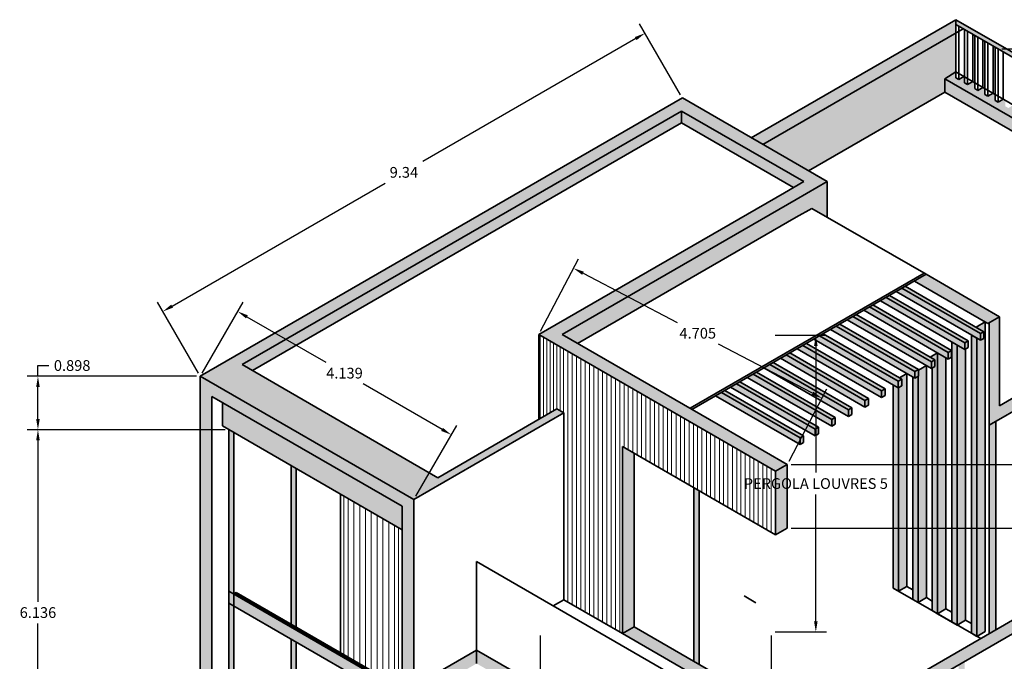
# Model space of a CAD drawing. Units: metres. Extents: x 26125 to 52281, y 14233 to 28508.
# Tile 3 of 4: x 26125.05 to 26141.57, y 14248.53 to 14259.3. Entities that reach past the tile are written whole.
import ezdxf

# ---------------------------------------------------------------- set-up
doc = ezdxf.new("R2010")
doc.units = ezdxf.units.M
for name, color, linetype, lineweight in [('A-ANNO-DIMS', 2, 'Continuous', 18), ('A-ELEV-CLAD', 30, 'Continuous', 13), ('A-ELEV-PATT', 32, 'Continuous', 13), ('A-WALL', 7, 'Continuous', 35), ('A-WALL-PATT', 9, 'Continuous', 13)]:
    doc.layers.add(name, color=color, linetype=linetype, lineweight=lineweight)
doc.styles.get("Standard").update_dxf_attribs({"font": 'arial.ttf'})
doc.dimstyles.get("Standard").update_dxf_attribs({"dimtxt": 0.18, "dimasz": 0.18, "dimexe": 0.18, "dimexo": 0.0625, "dimgap": 0.09, "dimtad": 0, "dimtih": 1, "dimtoh": 1, "dimdec": 4, "dimzin": 0, "dimdsep": 46, "dimtxsty": 'Standard', "dimcen": 0.09, "dimadec": 0, "dimazin": 0, "dimtfac": 1, "dimtdec": 4, "dimtofl": 0, "dimtmove": 0, "dimatfit": 3, "dimfxl": 1, "dimtolj": 1, "dimtzin": 0, "dimarcsym": 0})

# ---------------------------------------------------------------- blocks, each defined once
blk = doc.blocks.new('LINES')
for p, q in [((26133.777, 14254.006), (26133.777, 14252.604)), ((26133.833, 14253.974), (26133.833, 14252.637)), ((26133.889, 14253.942), (26133.889, 14252.669)), ((26133.945, 14253.91), (26133.945, 14252.701)), ((26134.001, 14253.877), (26134.001, 14252.733)), ((26134.057, 14253.845), (26134.057, 14252.766)), ((26134.112, 14253.813), (26134.112, 14252.738)), ((26134.168, 14253.781), (26134.168, 14252.706)), ((26134.241, 14253.739), (26134.241, 14249.53)), ((26134.314, 14253.697), (26134.314, 14249.488)), ((26134.386, 14253.655), (26134.386, 14249.446)), ((26134.459, 14253.613), (26134.459, 14249.404)), ((26134.532, 14253.571), (26134.532, 14249.362)), ((26134.604, 14253.529), (26134.604, 14249.32)), ((26134.677, 14253.487), (26134.677, 14249.278)), ((26134.75, 14253.445), (26134.75, 14249.236)), ((26134.822, 14253.403), (26134.822, 14249.194)), ((26134.895, 14253.361), (26134.895, 14249.152)), ((26134.968, 14253.319), (26134.968, 14249.111)), ((26135.04, 14253.277), (26135.04, 14249.069)), ((26135.113, 14253.235), (26135.113, 14249.027)), ((26135.186, 14253.193), (26135.186, 14252.124)), ((26135.258, 14253.151), (26135.258, 14252.082)), ((26135.331, 14253.109), (26135.331, 14252.04)), ((26135.404, 14253.067), (26135.404, 14251.998)), ((26135.477, 14253.025), (26135.477, 14251.956)), ((26135.549, 14252.983), (26135.549, 14251.914)), ((26135.622, 14252.941), (26135.622, 14251.872)), ((26135.695, 14252.899), (26135.695, 14251.83)), ((26135.767, 14252.857), (26135.767, 14251.788)), ((26135.84, 14252.815), (26135.84, 14251.746)), ((26135.913, 14252.774), (26135.913, 14251.704)), ((26135.985, 14252.732), (26135.985, 14251.662)), ((26136.058, 14252.69), (26136.058, 14251.62)), ((26136.131, 14252.648), (26136.131, 14251.578)), ((26136.203, 14252.606), (26136.203, 14251.536)), ((26136.276, 14252.564), (26136.276, 14251.494)), ((26136.349, 14252.522), (26136.349, 14251.452)), ((26136.421, 14252.48), (26136.421, 14251.41)), ((26136.494, 14252.438), (26136.494, 14251.368)), ((26136.567, 14252.396), (26136.567, 14251.326)), ((26136.639, 14252.354), (26136.639, 14251.284)), ((26136.712, 14252.312), (26136.712, 14251.242)), ((26136.785, 14252.27), (26136.785, 14251.2)), ((26136.857, 14252.228), (26136.857, 14251.158)), ((26136.93, 14252.186), (26136.93, 14251.116)), ((26137.003, 14252.144), (26137.003, 14251.074)), ((26137.076, 14252.102), (26137.076, 14251.033)), ((26137.148, 14252.06), (26137.148, 14250.991)), ((26137.221, 14252.018), (26137.221, 14250.949)), ((26137.294, 14251.976), (26137.294, 14250.907)), ((26137.366, 14251.934), (26137.366, 14250.865)), ((26137.439, 14251.892), (26137.439, 14250.823)), ((26137.512, 14251.85), (26137.512, 14250.781)), ((26137.584, 14251.808), (26137.584, 14250.739)), ((26137.657, 14251.766), (26137.657, 14250.697))]:
    blk.add_line(p, q)
blk = doc.blocks.new('*D8')
at = {"layer": 'A-ANNO-DIMS', "color": 0, "lineweight": -2, "transparency": 16777216}
for p, q in [((26137.719, 14254.006), (26138.584, 14254.006)), ((26138.404, 14253.826), (26138.404, 14251.7)), ((26138.404, 14249.207), (26138.404, 14251.333)), ((26137.719, 14249.027), (26138.584, 14249.027))]:
    blk.add_line(p, q, dxfattribs=at)
at = {"layer": 'A-ANNO-DIMS', "color": 0, "transparency": 16777216}
for points in [[(26138.374, 14253.826), (26138.434, 14253.826), (26138.404, 14254.006)], [(26138.374, 14249.207), (26138.434, 14249.207), (26138.404, 14249.027)]]:
    blk.add_solid(points, dxfattribs=at)
at = {"layer": 'Defpoints', "color": 0, "transparency": 16777216}
for p in [(26137.657, 14254.006), (26138.404, 14254.006), (26137.657, 14249.027)]:
    blk.add_point(p, dxfattribs=at)
at = {"layer": 'A-ANNO-DIMS', "color": 0, "transparency": 16777216, "insert": (26138.404, 14251.517), "char_height": 0.18, "attachment_point": 5}
blk.add_mtext('\\A1;PERGOLA LOUVRES 5', dxfattribs=at)
blk = doc.blocks.new('*D9')
at = {"layer": 'A-ANNO-DIMS', "color": 0, "lineweight": -2, "transparency": 16777216}
for p, q in [((26133.777, 14248.964), (26133.777, 14248.1)), ((26137.657, 14248.964), (26137.657, 14248.1)), ((26133.957, 14248.28), (26135.565, 14248.28)), ((26137.477, 14248.28), (26135.869, 14248.28))]:
    blk.add_line(p, q, dxfattribs=at)
at = {"layer": 'A-ANNO-DIMS', "color": 0, "transparency": 16777216}
for points in [[(26133.957, 14248.31), (26133.957, 14248.25), (26133.777, 14248.28)], [(26137.477, 14248.31), (26137.477, 14248.25), (26137.657, 14248.28)]]:
    blk.add_solid(points, dxfattribs=at)
at = {"layer": 'Defpoints', "color": 0, "transparency": 16777216}
for p in [(26133.777, 14249.027), (26137.657, 14249.027), (26137.657, 14248.28)]:
    blk.add_point(p, dxfattribs=at)
at = {"layer": 'A-ANNO-DIMS', "color": 0, "transparency": 16777216, "insert": (26135.717, 14248.28), "char_height": 0.18, "attachment_point": 5}
blk.add_mtext('\\A1;4', dxfattribs=at)
blk = doc.blocks.new('*D11')
at = {"layer": 'A-ANNO-DIMS', "color": 0, "lineweight": -2, "transparency": 16777216}
for p, q in [((26141.524, 14258.813), (26150.226, 14258.813)), ((26150.046, 14258.633), (26150.046, 14247.091)), ((26150.046, 14235.186), (26150.046, 14246.727)), ((26136.826, 14235.006), (26150.226, 14235.006))]:
    blk.add_line(p, q, dxfattribs=at)
at = {"layer": 'A-ANNO-DIMS', "color": 0, "transparency": 16777216}
for points in [[(26150.016, 14258.633), (26150.076, 14258.633), (26150.046, 14258.813)], [(26150.016, 14235.186), (26150.076, 14235.186), (26150.046, 14235.006)]]:
    blk.add_solid(points, dxfattribs=at)
at = {"layer": 'Defpoints', "color": 0, "transparency": 16777216}
for p in [(26141.462, 14258.813), (26150.046, 14258.813), (26136.763, 14235.006)]:
    blk.add_point(p, dxfattribs=at)
at = {"layer": 'A-ANNO-DIMS', "color": 0, "transparency": 16777216, "insert": (26150.046, 14246.909), "char_height": 0.18, "attachment_point": 5}
blk.add_mtext('\\A1;23.807', dxfattribs=at)
blk = doc.blocks.new('*D19')
at = {"layer": 'A-ANNO-DIMS', "color": 0, "lineweight": -2, "transparency": 16777216}
for p, q in [((26128.107, 14253.372), (26128.794, 14254.561)), ((26128.859, 14254.315), (26130.181, 14253.552)), ((26132.132, 14252.426), (26130.811, 14253.188)), ((26131.692, 14251.303), (26132.378, 14252.492))]:
    blk.add_line(p, q, dxfattribs=at)
at = {"layer": 'A-ANNO-DIMS', "color": 0, "transparency": 16777216}
for points in [[(26128.874, 14254.341), (26128.844, 14254.289), (26128.704, 14254.405)], [(26132.147, 14252.452), (26132.117, 14252.4), (26132.288, 14252.336)]]:
    blk.add_solid(points, dxfattribs=at)
at = {"layer": 'Defpoints', "color": 0, "transparency": 16777216}
for p in [(26128.076, 14253.318), (26132.288, 14252.336), (26131.66, 14251.249)]:
    blk.add_point(p, dxfattribs=at)
at = {"layer": 'A-ANNO-DIMS', "color": 0, "transparency": 16777216, "insert": (26130.496, 14253.37), "char_height": 0.18, "attachment_point": 5}
blk.add_mtext('\\A1;4.139', dxfattribs=at)
blk = doc.blocks.new('*D20')
at = {"layer": 'A-ANNO-DIMS', "color": 0, "lineweight": -2, "transparency": 16777216}
for p, q in [((26136.134, 14258.043), (26135.447, 14259.231)), ((26135.382, 14258.985), (26131.808, 14256.922)), ((26127.604, 14254.495), (26131.178, 14256.558)), ((26128.045, 14253.372), (26127.359, 14254.561))]:
    blk.add_line(p, q, dxfattribs=at)
at = {"layer": 'A-ANNO-DIMS', "color": 0, "transparency": 16777216}
for points in [[(26135.367, 14259.011), (26135.397, 14258.959), (26135.537, 14259.075)], [(26127.589, 14254.521), (26127.619, 14254.469), (26127.449, 14254.405)]]:
    blk.add_solid(points, dxfattribs=at)
at = {"layer": 'Defpoints', "color": 0, "transparency": 16777216}
for p in [(26135.537, 14259.075), (26136.165, 14257.988), (26128.076, 14253.318)]:
    blk.add_point(p, dxfattribs=at)
at = {"layer": 'A-ANNO-DIMS', "color": 0, "transparency": 16777216, "insert": (26131.493, 14256.74), "char_height": 0.18, "attachment_point": 5}
blk.add_mtext('\\A1;9.34', dxfattribs=at)
blk = doc.blocks.new('*D21')
at = {"layer": 'A-ANNO-DIMS', "color": 0, "lineweight": -2, "transparency": 16777216}
for p, q in [((26133.786, 14254.074), (26134.422, 14255.29)), ((26134.498, 14255.047), (26136.075, 14254.222)), ((26138.348, 14253.033), (26136.77, 14253.858)), ((26137.954, 14251.893), (26138.591, 14253.109))]:
    blk.add_line(p, q, dxfattribs=at)
at = {"layer": 'A-ANNO-DIMS', "color": 0, "transparency": 16777216}
for points in [[(26134.512, 14255.073), (26134.484, 14255.02), (26134.338, 14255.13)], [(26138.362, 14253.06), (26138.334, 14253.006), (26138.507, 14252.949)]]:
    blk.add_solid(points, dxfattribs=at)
at = {"layer": 'Defpoints', "color": 0, "transparency": 16777216}
for p in [(26133.757, 14254.018), (26138.507, 14252.949), (26137.925, 14251.837)]:
    blk.add_point(p, dxfattribs=at)
at = {"layer": 'A-ANNO-DIMS', "color": 0, "transparency": 16777216, "insert": (26136.423, 14254.04), "char_height": 0.18, "attachment_point": 5}
blk.add_mtext('\\A1;4.705', dxfattribs=at)
blk = doc.blocks.new('*D22')
at = {"layer": 'A-ANNO-DIMS', "color": 0, "lineweight": -2, "transparency": 16777216}
for p, q in [((26137.988, 14251.837), (26150.226, 14251.837)), ((26150.046, 14251.657), (26150.046, 14251.485)), ((26150.046, 14250.948), (26150.046, 14251.121)), ((26137.988, 14250.768), (26150.226, 14250.768))]:
    blk.add_line(p, q, dxfattribs=at)
at = {"layer": 'A-ANNO-DIMS', "color": 0, "transparency": 16777216}
for points in [[(26150.016, 14251.657), (26150.076, 14251.657), (26150.046, 14251.837)], [(26150.016, 14250.948), (26150.076, 14250.948), (26150.046, 14250.768)]]:
    blk.add_solid(points, dxfattribs=at)
at = {"layer": 'Defpoints', "color": 0, "transparency": 16777216}
for p in [(26137.925, 14251.837), (26137.925, 14250.768), (26150.046, 14250.768)]:
    blk.add_point(p, dxfattribs=at)
at = {"layer": 'A-ANNO-DIMS', "color": 0, "transparency": 16777216, "insert": (26150.046, 14251.303), "char_height": 0.18, "attachment_point": 5}
blk.add_mtext('\\A1;1.07', dxfattribs=at)
blk = doc.blocks.new('*D26')
at = {"layer": 'A-ANNO-DIMS', "color": 0, "lineweight": -2, "transparency": 16777216}
for p, q in [((26128.496, 14252.42), (26125.173, 14252.42)), ((26125.353, 14252.24), (26125.353, 14249.534)), ((26125.353, 14246.464), (26125.353, 14249.17)), ((26128.496, 14246.284), (26125.173, 14246.284))]:
    blk.add_line(p, q, dxfattribs=at)
at = {"layer": 'A-ANNO-DIMS', "color": 0, "transparency": 16777216}
for points in [[(26125.323, 14252.24), (26125.383, 14252.24), (26125.353, 14252.42)], [(26125.323, 14246.464), (26125.383, 14246.464), (26125.353, 14246.284)]]:
    blk.add_solid(points, dxfattribs=at)
at = {"layer": 'Defpoints', "color": 0, "transparency": 16777216}
for p in [(26125.353, 14252.42), (26128.558, 14252.42), (26128.558, 14246.284)]:
    blk.add_point(p, dxfattribs=at)
at = {"layer": 'A-ANNO-DIMS', "color": 0, "transparency": 16777216, "insert": (26125.353, 14249.352), "char_height": 0.18, "attachment_point": 5}
blk.add_mtext('\\A1;6.136', dxfattribs=at)
blk = doc.blocks.new('*D27')
at = {"layer": 'A-ANNO-DIMS', "color": 0, "lineweight": -2, "transparency": 16777216}
for p, q in [((26125.353, 14253.318), (26125.353, 14253.498)), ((26125.353, 14253.498), (26125.533, 14253.498)), ((26128.014, 14253.318), (26125.173, 14253.318)), ((26125.353, 14252.6), (26125.353, 14253.138)), ((26128.496, 14252.42), (26125.173, 14252.42))]:
    blk.add_line(p, q, dxfattribs=at)
at = {"layer": 'A-ANNO-DIMS', "color": 0, "transparency": 16777216}
for points in [[(26125.323, 14253.138), (26125.383, 14253.138), (26125.353, 14253.318)], [(26125.323, 14252.6), (26125.383, 14252.6), (26125.353, 14252.42)]]:
    blk.add_solid(points, dxfattribs=at)
at = {"layer": 'Defpoints', "color": 0, "transparency": 16777216}
for p in [(26125.353, 14253.318), (26128.076, 14253.318), (26128.558, 14252.42)]:
    blk.add_point(p, dxfattribs=at)
at = {"layer": 'A-ANNO-DIMS', "color": 0, "transparency": 16777216, "insert": (26125.927, 14253.498), "char_height": 0.18, "attachment_point": 5}
blk.add_mtext('\\A1;0.898', dxfattribs=at)

msp = doc.modelspace()

# ---------------------------------------------------------------- hatches: boundary and pattern name
at = {"layer": 'A-ELEV-PATT'}
h = msp.add_hatch(color=256, dxfattribs=at)
h.dxf.hatch_style = 1
h.paths.add_polyline_path([(26140.2525, 14255.0285), (26140.2206, 14255.0469), (26136.2935, 14252.7796), (26136.3254, 14252.7612)])
h = msp.add_hatch(color=256, dxfattribs=at)
h.dxf.hatch_style = 1
h.paths.add_polyline_path([(26137.9664, 14253.7086), (26137.9088, 14253.6753), (26139.2286, 14252.9133), (26139.2862, 14252.9466)])
h.paths.add_polyline_path([(26137.9088, 14253.6753), (26137.8118, 14253.6194), (26139.2286, 14252.8014), (26139.2286, 14252.9133)])
h.paths.add_polyline_path([(26139.2862, 14252.9466), (26139.2286, 14252.9133), (26139.2286, 14252.8014), (26139.2862, 14252.8347)])
h.paths.add_polyline_path([(26139.5077, 14253.0745), (26138.1879, 14253.8365), (26138.091, 14253.7805), (26139.5077, 14252.9626)])
h.paths.add_polyline_path([(26138.2456, 14253.8698), (26138.1879, 14253.8365), (26139.5077, 14253.0745), (26139.5654, 14253.1078)])
h.paths.add_polyline_path([(26139.5654, 14253.1078), (26139.5077, 14253.0745), (26139.5077, 14252.9626), (26139.5654, 14252.9959)])
h.paths.add_polyline_path([(26138.467, 14253.9977), (26138.3701, 14253.9417), (26139.7869, 14253.1237), (26139.7869, 14253.2357)])
h.paths.add_polyline_path([(26138.5247, 14254.0309), (26138.467, 14253.9977), (26139.7869, 14253.2357), (26139.8445, 14253.2689)])
h.paths.add_polyline_path([(26139.8445, 14253.2689), (26139.7869, 14253.2357), (26139.7869, 14253.1237), (26139.8445, 14253.157)])
h.paths.add_polyline_path([(26140.1237, 14253.4301), (26140.066, 14253.3968), (26140.066, 14253.2849), (26140.1237, 14253.3182)])
h.paths.add_polyline_path([(26138.8038, 14254.1921), (26138.7462, 14254.1588), (26140.066, 14253.3968), (26140.1237, 14253.4301)])
h.paths.add_polyline_path([(26138.7462, 14254.1588), (26138.6493, 14254.1029), (26140.066, 14253.2849), (26140.066, 14253.3968)])
h.paths.add_polyline_path([(26139.0253, 14254.32), (26138.9284, 14254.264), (26140.3451, 14253.4461), (26140.3451, 14253.558)])
h.paths.add_polyline_path([(26139.083, 14254.3533), (26139.0253, 14254.32), (26140.3451, 14253.558), (26140.4028, 14253.5913)])
h.paths.add_polyline_path([(26140.4028, 14253.5913), (26140.3451, 14253.558), (26140.3451, 14253.4461), (26140.4028, 14253.4793)])
h.paths.add_polyline_path([(26139.3045, 14254.4811), (26139.2075, 14254.4252), (26140.6243, 14253.6072), (26140.6243, 14253.7191)])
h.paths.add_polyline_path([(26139.3621, 14254.5144), (26139.3045, 14254.4811), (26140.6243, 14253.7191), (26140.6819, 14253.7524)])
h.paths.add_polyline_path([(26140.6819, 14253.7524), (26140.6243, 14253.7191), (26140.6243, 14253.6072), (26140.6819, 14253.6405)])
h.paths.add_polyline_path([(26139.5836, 14254.6423), (26139.4867, 14254.5863), (26140.9034, 14253.7684), (26140.9034, 14253.8803)])
h.paths.add_polyline_path([(26139.6412, 14254.6756), (26139.5836, 14254.6423), (26140.9034, 14253.8803), (26140.9611, 14253.9136)])
h.paths.add_polyline_path([(26140.9611, 14253.9136), (26140.9034, 14253.8803), (26140.9034, 14253.7684), (26140.9611, 14253.8017)])
h.paths.add_polyline_path([(26139.8476, 14254.7947), (26139.7506, 14254.7387), (26141.1674, 14253.9208), (26141.1674, 14254.0327)])
h.paths.add_polyline_path([(26139.9052, 14254.828), (26139.8476, 14254.7947), (26141.1674, 14254.0327), (26141.225, 14254.066)])
h.paths.add_polyline_path([(26141.225, 14254.066), (26141.1674, 14254.0327), (26141.1674, 14253.9208), (26141.225, 14253.9541)])
h = msp.add_hatch(color=256, dxfattribs=at)
h.dxf.hatch_style = 1
h.paths.add_polyline_path([(26141.2443, 14254.2299), (26141.0927, 14254.1424), (26141.225, 14254.066), (26141.225, 14253.9541), (26141.1674, 14253.9208), (26141.1045, 14253.9571), (26141.1045, 14249.1138), (26141.2443, 14249.0331)])
h.paths.add_polyline_path([(26141.2443, 14249.0331), (26141.1045, 14249.1138), (26141.1045, 14248.9523)])
h.paths.add_polyline_path([(26141.1045, 14253.9571), (26141.015, 14254.0088), (26141.015, 14249.004), (26141.1045, 14248.9523), (26141.1045, 14249.1138)])
h.paths.add_polyline_path([(26141.4248, 14252.5622), (26141.3093, 14252.4955), (26141.3093, 14248.9955), (26141.4248, 14249.0622)])
h.paths.add_polyline_path([(26140.9159, 14253.7756), (26140.9034, 14253.7684), (26140.7761, 14253.8419), (26140.7761, 14249.3033), (26140.9159, 14249.2226)])
h.paths.add_polyline_path([(26140.7761, 14253.8419), (26140.6854, 14253.8942), (26140.6854, 14249.1943), (26140.7761, 14249.1419)])
h.paths.add_polyline_path([(26140.9159, 14249.2226), (26140.7761, 14249.3033), (26140.7761, 14249.1419)])
h.paths.add_polyline_path([(26140.4478, 14249.4929), (26140.4478, 14249.3315), (26140.5876, 14249.4122)])
h.paths.add_polyline_path([(26140.5876, 14253.6284), (26140.4478, 14253.7091), (26140.4478, 14249.4929), (26140.5876, 14249.4122)])
h.paths.add_polyline_path([(26140.4478, 14253.7091), (26140.3232, 14253.6372), (26140.4028, 14253.5913), (26140.4028, 14253.4793), (26140.3571, 14253.4529), (26140.3571, 14249.3839), (26140.4478, 14249.3315), (26140.4478, 14249.4929)])
h.paths.add_polyline_path([(26140.2592, 14253.4957), (26140.1237, 14253.4174), (26140.1237, 14253.3182), (26140.1194, 14253.3157), (26140.1194, 14249.6825), (26140.2592, 14249.6018)])
h.paths.add_polyline_path([(26140.1194, 14253.3157), (26140.066, 14253.2849), (26140.0287, 14253.3064), (26140.0287, 14249.5735), (26140.1194, 14249.5211)])
h.paths.add_polyline_path([(26140.1194, 14249.6825), (26140.1194, 14249.5211), (26140.2592, 14249.6018)])
h = msp.add_hatch(color=256, dxfattribs=at)
h.dxf.hatch_style = 1
h.paths.add_polyline_path([(26136.8199, 14253.0467), (26136.723, 14252.9907), (26138.1397, 14252.1728), (26138.1397, 14252.2847)])
h.paths.add_polyline_path([(26136.8776, 14253.08), (26136.8199, 14253.0467), (26138.1397, 14252.2847), (26138.1974, 14252.318)])
h.paths.add_polyline_path([(26138.1974, 14252.318), (26138.1397, 14252.2847), (26138.1397, 14252.1728), (26138.1974, 14252.206)])
h.paths.add_polyline_path([(26137.0714, 14253.1918), (26136.9744, 14253.1359), (26138.3912, 14252.3179), (26138.3912, 14252.4298)])
h.paths.add_polyline_path([(26137.129, 14253.2251), (26137.0714, 14253.1918), (26138.3912, 14252.4298), (26138.4488, 14252.4631)])
h.paths.add_polyline_path([(26138.4488, 14252.4631), (26138.3912, 14252.4298), (26138.3912, 14252.3179), (26138.4488, 14252.3512)])
h.paths.add_polyline_path([(26137.3505, 14253.353), (26137.2536, 14253.2971), (26138.6703, 14252.4791), (26138.6703, 14252.591)])
h.paths.add_polyline_path([(26137.4081, 14253.3863), (26137.3505, 14253.353), (26138.6703, 14252.591), (26138.728, 14252.6243)])
h.paths.add_polyline_path([(26138.728, 14252.6243), (26138.6703, 14252.591), (26138.6703, 14252.4791), (26138.728, 14252.5124)])
h.paths.add_polyline_path([(26137.6296, 14253.5142), (26137.5327, 14253.4582), (26138.9495, 14252.6403), (26138.9495, 14252.7522)])
h.paths.add_polyline_path([(26137.6873, 14253.5475), (26137.6296, 14253.5142), (26138.9495, 14252.7522), (26139.0071, 14252.7855)])
h.paths.add_polyline_path([(26139.0071, 14252.7855), (26138.9495, 14252.7522), (26138.9495, 14252.6403), (26139.0071, 14252.6735)])
h = msp.add_hatch(color=256, dxfattribs=at)
h.dxf.hatch_style = 1
h.paths.add_polyline_path([(26139.791, 14253.1261), (26139.7869, 14253.1237), (26139.7003, 14253.1737), (26139.7003, 14249.763), (26139.791, 14249.7107)])
h.paths.add_polyline_path([(26139.9308, 14253.3629), (26139.8063, 14253.291), (26139.8445, 14253.2689), (26139.8445, 14253.157), (26139.791, 14253.1261), (26139.791, 14249.7107), (26139.9308, 14249.7914)])
h = msp.add_hatch(color=256, dxfattribs=at)
h.dxf.hatch_style = 1
h.paths.add_polyline_path([(26139.7617, 14247.876), (26139.6635, 14247.8193), (26139.6635, 14244.3193), (26139.7617, 14244.376)])
h.paths.add_polyline_path([(26134.1363, 14247.6744), (26134.0497, 14247.7244), (26134.0497, 14244.7066), (26134.1363, 14244.7566)])
h.paths.add_polyline_path([(26135.2033, 14244.0405), (26135.3053, 14244.1136), (26135.3053, 14246.9994), (26135.2033, 14247.0583)])
h.paths.add_polyline_path([(26140.8009, 14238.75), (26140.8988, 14238.8065), (26140.8988, 14244.8065), (26140.8009, 14244.75)])
h.paths.add_polyline_path([(26142.7463, 14245.8732), (26142.6308, 14245.8065), (26142.6308, 14239.8065), (26142.7463, 14239.8732)])
h.paths.add_polyline_path([(26142.7463, 14249.5992), (26142.6308, 14249.5325), (26142.6308, 14246.0325), (26142.7463, 14246.0992)])
h.paths.add_polyline_path([(26140.8009, 14244.976), (26140.8988, 14245.0325), (26140.8988, 14248.5325), (26140.8009, 14248.476)])
h.paths.add_polyline_path([(26142.6308, 14249.7585), (26142.7463, 14249.8252), (26142.7463, 14253.3252), (26142.6308, 14253.2585)])
h.paths.add_polyline_path([(26136.4442, 14251.397), (26136.3576, 14251.447), (26136.3576, 14248.5341), (26136.4442, 14248.4841)])
h = msp.add_hatch(color=256, dxfattribs=at)
h.dxf.hatch_style = 1
h.paths.add_polyline_path([(26128.4472, 14252.878), (26128.4472, 14252.4843), (26131.4647, 14250.7421), (26131.4647, 14251.1359)])
h = msp.add_hatch(color=256, dxfattribs=at)
h.dxf.hatch_style = 1
h.paths.add_polyline_path([(26128.6368, 14249.6632), (26128.6368, 14249.4632), (26131.4647, 14247.8305), (26131.4647, 14248.0305)])
h.paths.add_polyline_path([(26129.6878, 14248.8564), (26129.5992, 14248.9076), (26129.5992, 14245.7744), (26129.6878, 14245.7232)])
h.paths.add_polyline_path([(26128.6368, 14249.4632), (26128.558, 14249.5087), (26128.558, 14246.2845), (26128.6368, 14246.33)])
h.paths.add_polyline_path([(26128.6368, 14249.6632), (26128.558, 14249.7087), (26128.558, 14249.5087), (26128.6368, 14249.4632)])
h.paths.add_polyline_path([(26128.6368, 14252.3748), (26128.558, 14252.4203), (26128.558, 14249.7087), (26128.6368, 14249.6632)])
h.paths.add_polyline_path([(26128.651, 14245.2941), (26128.5813, 14245.3344), (26128.5813, 14241.8829), (26128.651, 14241.9232)])
h.paths.add_polyline_path([(26128.651, 14241.9232), (26128.5813, 14241.8829), (26129.4364, 14241.3893), (26129.4364, 14241.4697)])
h.paths.add_polyline_path([(26129.4797, 14241.4143), (26129.4364, 14241.3893), (26130.2914, 14240.8956), (26130.2914, 14240.9456)])
h.paths.add_polyline_path([(26130.3373, 14240.9221), (26130.2914, 14240.8956), (26131.1464, 14240.402), (26131.1464, 14240.455)])
h.paths.add_polyline_path([(26130.3373, 14244.3206), (26130.2914, 14244.3471), (26130.2914, 14240.8956), (26130.3373, 14240.9221)])
h.paths.add_polyline_path([(26129.4797, 14244.8157), (26129.4364, 14244.8407), (26129.4364, 14241.3893), (26129.4797, 14241.4143)])
h.paths.add_polyline_path([(26135.2508, 14242.6282), (26135.1411, 14242.6915), (26135.1411, 14239.2275), (26135.2508, 14239.2908)])
h.paths.add_polyline_path([(26133.8091, 14243.4606), (26133.706, 14243.5201), (26133.706, 14240.056), (26133.8091, 14240.1155)])
h.paths.add_polyline_path([(26132.3223, 14244.3189), (26132.2523, 14244.2785), (26132.2523, 14240.7692), (26132.3223, 14240.7288)])
h = msp.add_hatch(color=256, dxfattribs=at)
h.dxf.hatch_style = 1
h.paths.add_polyline_path([(26129.6878, 14251.768), (26129.5992, 14251.8192), (26129.5992, 14249.1586), (26129.6878, 14249.1074)])
at = {"layer": 'A-WALL-PATT'}
h = msp.add_hatch(color=256, dxfattribs=at)
h.dxf.hatch_style = 1
h.paths.add_polyline_path([(26132.7127, 14248.4963), (26132.7127, 14248.7223), (26131.6604, 14248.1148), (26131.6604, 14247.8888)])
h.paths.add_polyline_path([(26132.7127, 14248.7223), (26132.7127, 14248.4963), (26136.7743, 14246.1513), (26136.7743, 14246.3773)])
h.paths.add_polyline_path([(26145.7774, 14251.3492), (26145.7774, 14250.8522), (26145.9732, 14250.9652), (26145.9732, 14251.6882), (26145.9732, 14252.3156), (26145.7774, 14252.4288), (26145.7774, 14251.5752), (26136.7743, 14246.3773), (26136.7743, 14246.1513), (26136.97, 14246.2643), (26136.97, 14246.1509), (26137.1658, 14246.2639), (26137.1658, 14246.3773)])
h.paths.add_polyline_path([(26135.3545, 14249.1132), (26135.1588, 14249.0002), (26138.2381, 14247.2224), (26138.4338, 14247.3354)])
h.paths.add_polyline_path([(26135.3545, 14252.0261), (26135.1588, 14252.1391), (26135.1588, 14249.0002), (26135.3545, 14249.1132)])
h.paths.add_polyline_path([(26137.9254, 14251.8375), (26137.7296, 14251.7245), (26137.7296, 14250.6548), (26137.9254, 14250.7678)], flags=17)
h.paths.add_polyline_path([(26144.9726, 14252.8939), (26144.9726, 14254.6106), (26144.7764, 14254.4973), (26144.7764, 14252.7806), (26145.7774, 14252.2026), (26145.7774, 14252.4288)])
h.paths.add_polyline_path([(26147.5095, 14248.6232), (26147.5095, 14242.6232), (26147.7052, 14242.7362), (26147.7052, 14248.9622), (26136.1883, 14242.3129), (26136.1883, 14242.0869), (26136.97, 14242.5383), (26136.97, 14242.3123), (26137.1658, 14242.4253), (26137.1658, 14242.6513)])
h.paths.add_polyline_path([(26145.9732, 14249.2872), (26145.7774, 14249.1742), (26145.7774, 14247.8492), (26145.9732, 14247.9622)], flags=17)
h.paths.add_polyline_path([(26145.5817, 14254.9622), (26145.5817, 14254.7362), (26145.7774, 14254.8492), (26145.7774, 14255.5272), (26145.5817, 14255.4142), (26145.5817, 14255.1882), (26141.4857, 14252.8234), (26141.4857, 14252.5974)])
h.paths.add_polyline_path([(26140.5667, 14258.3096), (26140.5667, 14258.0836), (26145.5817, 14255.1882), (26145.5817, 14255.4142)])
h.paths.add_polyline_path([(26140.7524, 14259.0772), (26140.7524, 14259.3025), (26137.3207, 14257.3212), (26137.5157, 14257.2086)])
h.paths.add_polyline_path([(26138.0751, 14255.9856), (26138.3349, 14256.1356), (26138.5947, 14255.9856), (26138.5947, 14256.5856), (26138.0751, 14256.2856), (26134.148, 14254.0183), (26134.4078, 14253.8683)])
h.paths.add_polyline_path([(26140.5667, 14258.0836), (26140.5667, 14258.3096), (26140.7524, 14258.4285), (26140.7524, 14259.0772), (26137.5157, 14257.2086), (26138.2834, 14256.7653)])
h.paths.add_polyline_path([(26145.1083, 14255.9136), (26145.0216, 14255.8636), (26144.9721, 14255.8922), (26144.9721, 14255.9922), (26144.9373, 14256.0123), (26144.8507, 14255.9623), (26144.8012, 14255.9909), (26144.8012, 14256.0909), (26144.7664, 14256.1109), (26144.6798, 14256.0609), (26144.6303, 14256.0896), (26144.6303, 14256.1896), (26144.5955, 14256.2096), (26144.5089, 14256.1596), (26144.4594, 14256.1882), (26144.4594, 14256.2882), (26144.4246, 14256.3083), (26144.338, 14256.2583), (26144.2885, 14256.2869), (26144.2885, 14256.3869), (26144.2537, 14256.407), (26144.1671, 14256.357), (26144.1176, 14256.3856), (26144.1176, 14256.4856), (26144.0828, 14256.5056), (26143.9962, 14256.4556), (26143.9466, 14256.4842), (26143.9466, 14256.5842), (26143.9119, 14256.6043), (26143.8253, 14256.5543), (26143.7757, 14256.5829), (26143.7757, 14256.6829), (26143.741, 14256.703), (26143.6544, 14256.653), (26143.6048, 14256.6816), (26143.6048, 14256.7816), (26143.5701, 14256.8017), (26143.4835, 14256.7517), (26143.4339, 14256.7803), (26143.4339, 14256.8803), (26143.3992, 14256.9003), (26143.3126, 14256.8503), (26143.263, 14256.8789), (26143.263, 14256.9789), (26143.2283, 14256.999), (26143.1417, 14256.949), (26143.0921, 14256.9776), (26143.0921, 14257.0776), (26143.0573, 14257.0977), (26142.9707, 14257.0477), (26142.9212, 14257.0763), (26142.9212, 14257.1763), (26142.8864, 14257.1964), (26142.7998, 14257.1464), (26142.7503, 14257.175), (26142.7503, 14257.275), (26142.7155, 14257.295), (26142.6289, 14257.245), (26142.5794, 14257.2736), (26142.5794, 14257.3736), (26142.5446, 14257.3937), (26142.458, 14257.3437), (26142.4085, 14257.3723), (26142.4085, 14257.4723), (26142.3737, 14257.4924), (26142.2871, 14257.4424), (26142.2376, 14257.471), (26142.2376, 14257.571), (26142.2322, 14257.5741), (26142.1456, 14257.5241), (26142.0961, 14257.5527), (26142.0961, 14257.6527), (26142.0613, 14257.6727), (26141.9747, 14257.6227), (26141.9252, 14257.6514), (26141.9252, 14257.7514), (26141.8904, 14257.7714), (26141.8038, 14257.7214), (26141.7542, 14257.75), (26141.7542, 14257.85), (26141.7195, 14257.8701), (26141.6329, 14257.8201), (26141.5833, 14257.8487), (26141.5833, 14257.9487), (26141.5486, 14257.9688), (26141.462, 14257.9188), (26141.4124, 14257.9474), (26141.4124, 14258.0474), (26141.3777, 14258.0674), (26141.2911, 14258.0174), (26141.2415, 14258.0461), (26141.2415, 14258.1461), (26141.2068, 14258.1661), (26141.1202, 14258.1161), (26141.0706, 14258.1447), (26141.0706, 14258.2447), (26141.0359, 14258.2648), (26140.9493, 14258.2148), (26140.8997, 14258.2434), (26140.8997, 14258.3434), (26140.8885, 14258.3499), (26140.8019, 14258.2999), (26140.7524, 14258.3285), (26140.7524, 14258.4285), (26140.5667, 14258.3096), (26145.5817, 14255.4142), (26145.7774, 14255.5272)])
h.paths.add_polyline_path([(26141.4857, 14254.3165), (26141.3093, 14254.2146), (26141.3093, 14252.4955), (26141.4857, 14252.5974)])
h.paths.add_polyline_path([(26140.2525, 14255.0285), (26140.0568, 14254.9155), (26141.29, 14254.2035), (26141.4857, 14254.3165)])
h = msp.add_hatch(color=256, dxfattribs=at)
h.dxf.hatch_style = 1
h.paths.add_polyline_path([(26140.7524, 14259.3025), (26140.7524, 14259.2223), (26145.0216, 14256.7575), (26145.1083, 14256.7876)])
h = msp.add_hatch(color=256, dxfattribs=at)
h.dxf.hatch_style = 1
h.paths.add_polyline_path([(26136.165, 14257.9884), (26128.0761, 14253.3183), (26131.6604, 14251.2489), (26134.1764, 14252.7015), (26134.0609, 14252.7682), (26132.0645, 14251.6156), (26128.7792, 14253.5123), (26136.1528, 14257.7695), (26138.2033, 14256.5856), (26137.8794, 14256.3986), (26133.7566, 14254.0183), (26137.7296, 14251.7245), (26137.9254, 14251.8375), (26136.7659, 14252.5069), (26134.148, 14254.0183), (26138.0751, 14256.2856), (26138.5947, 14256.5856)])
h = msp.add_hatch(color=256, dxfattribs=at)
h.dxf.hatch_style = 1
h.paths.add_polyline_path([(26136.1528, 14257.7695), (26136.1528, 14257.5695), (26138.0301, 14256.4856), (26138.2033, 14256.5856)])
h.paths.add_polyline_path([(26136.1528, 14257.5695), (26136.1528, 14257.7695), (26128.7792, 14253.5123), (26128.9524, 14253.4123)])
h = msp.add_hatch(color=256, dxfattribs=at)
h.dxf.hatch_style = 1
h.paths.add_polyline_path([(26131.6604, 14251.2489), (26128.0761, 14253.3183), (26128.0761, 14246.0062), (26131.6604, 14243.9368), (26131.6604, 14244.1628), (26128.2718, 14246.1192), (26128.2718, 14252.9793), (26131.4647, 14251.1359), (26131.4647, 14248.0305), (26131.6604, 14247.9175)])
h.paths.add_polyline_path([(26131.6604, 14245.2298), (26131.6604, 14247.7175), (26131.4647, 14247.8305), (26131.4647, 14244.2758), (26131.6604, 14244.1628)], flags=17)

# ---------------------------------------------------------------- linework, layer by layer
at = {"layer": 'A-ELEV-CLAD'}
for p, q in [((26130.4876, 14248.6456), (26130.4876, 14251.3062)), ((26130.5552, 14248.6066), (26130.5552, 14251.2672)), ((26130.6529, 14248.5502), (26130.6529, 14251.2108)), ((26130.7506, 14248.4938), (26130.7506, 14251.1544)), ((26130.8482, 14248.4374), (26130.8482, 14251.098)), ((26130.9459, 14248.381), (26130.9459, 14251.0416)), ((26131.0436, 14248.3246), (26131.0436, 14250.9853)), ((26131.1412, 14248.2682), (26131.1412, 14250.9289)), ((26131.2389, 14248.2118), (26131.2389, 14250.8725)), ((26131.3366, 14248.1554), (26131.3366, 14250.8161)), ((26131.3997, 14248.119), (26131.3997, 14250.7796))]:
    msp.add_line(p, q, dxfattribs=at)
at = {"layer": 'A-WALL'}
for p, q in [((26140.7524, 14259.3025), (26137.3207, 14257.3212)), ((26140.7524, 14258.3285), (26140.7524, 14259.3025)), ((26140.7524, 14259.3025), (26145.1083, 14256.7876)), ((26137.5157, 14257.2086), (26140.878, 14259.1498)), ((26140.7524, 14259.2223), (26145.0216, 14256.7575)), ((26140.8019, 14258.2999), (26140.8019, 14259.1937)), ((26140.8997, 14258.2434), (26140.8997, 14259.1373)), ((26140.9493, 14258.2148), (26140.9493, 14259.1087)), ((26141.0359, 14258.2648), (26141.0359, 14259.0587)), ((26141.0706, 14258.1447), (26141.0706, 14259.0386)), ((26141.1202, 14258.1161), (26141.1202, 14259.01)), ((26141.2068, 14258.1661), (26141.2068, 14258.96)), ((26141.2415, 14258.0461), (26141.2415, 14258.9399)), ((26141.2911, 14258.0174), (26141.2911, 14258.9113)), ((26141.3777, 14258.0674), (26141.3777, 14258.8613)), ((26141.4124, 14257.9474), (26141.4124, 14258.8413)), ((26141.462, 14257.9188), (26141.462, 14258.8126)), ((26141.5486, 14257.9688), (26141.5486, 14258.7626)), ((26140.7524, 14258.4285), (26140.5667, 14258.3096)), ((26140.5667, 14258.3096), (26145.5817, 14255.4142)), ((26140.5667, 14258.3096), (26140.5667, 14258.0836)), ((26145.7774, 14255.5272), (26140.7524, 14258.4285)), ((26140.8019, 14258.2999), (26140.7524, 14258.3285)), ((26140.8885, 14258.3499), (26140.8019, 14258.2999)), ((26140.9493, 14258.2148), (26140.8997, 14258.2434)), ((26141.0359, 14258.2648), (26140.9493, 14258.2148)), ((26141.1202, 14258.1161), (26141.0706, 14258.1447)), ((26141.2068, 14258.1661), (26141.1202, 14258.1161)), ((26136.165, 14257.9884), (26128.0761, 14253.3183)), ((26138.5947, 14256.5856), (26136.165, 14257.9884)), ((26140.5667, 14258.0836), (26138.2834, 14256.7653)), ((26145.5817, 14255.1882), (26140.5667, 14258.0836)), ((26141.2911, 14258.0174), (26141.2415, 14258.0461)), ((26141.3777, 14258.0674), (26141.2911, 14258.0174)), ((26141.462, 14257.9188), (26141.4124, 14257.9474)), ((26141.5486, 14257.9688), (26141.462, 14257.9188)), ((26136.1528, 14257.7695), (26128.7792, 14253.5123)), ((26138.2033, 14256.5856), (26136.1528, 14257.7695)), ((26136.1528, 14257.7695), (26136.1528, 14257.5695)), ((26136.1528, 14257.5695), (26128.9524, 14253.4123)), ((26138.0301, 14256.4856), (26136.1528, 14257.5695)), ((26138.5947, 14256.5856), (26138.399, 14256.6986)), ((26138.2033, 14256.5856), (26137.8794, 14256.3986)), ((26138.0751, 14256.2856), (26138.5947, 14256.5856)), ((26138.5947, 14256.5856), (26138.5947, 14255.9856)), ((26137.8794, 14256.3986), (26133.7566, 14254.0183)), ((26134.148, 14254.0183), (26138.0751, 14256.2856)), ((26138.0751, 14255.9856), (26138.3349, 14256.1356)), ((26140.2525, 14255.0285), (26138.3349, 14256.1356)), ((26134.4078, 14253.8683), (26138.0751, 14255.9856)), ((26141.4857, 14252.8234), (26145.5817, 14255.1882)), ((26140.2206, 14255.0469), (26136.2935, 14252.7796)), ((26140.2525, 14255.0285), (26136.3254, 14252.7612)), ((26141.4857, 14254.3165), (26140.2525, 14255.0285)), ((26140.0568, 14254.9155), (26141.29, 14254.2035)), ((26141.3093, 14252.4955), (26145.5817, 14254.9622)), ((26139.6412, 14254.6756), (26140.9611, 14253.9136)), ((26141.1674, 14253.9208), (26139.7506, 14254.7387)), ((26141.1674, 14254.0327), (26139.8476, 14254.7947)), ((26139.9052, 14254.828), (26141.225, 14254.066)), ((26139.3621, 14254.5144), (26140.6819, 14253.7524)), ((26140.9034, 14253.7684), (26139.4867, 14254.5863)), ((26140.9034, 14253.8803), (26139.5836, 14254.6423)), ((26139.083, 14254.3533), (26140.4028, 14253.5913)), ((26140.6243, 14253.6072), (26139.2075, 14254.4252)), ((26140.6243, 14253.7191), (26139.3045, 14254.4811)), ((26138.8038, 14254.1921), (26140.1237, 14253.4301)), ((26140.3451, 14253.4461), (26138.9284, 14254.264)), ((26140.3451, 14253.558), (26139.0253, 14254.32)), ((26141.2443, 14254.2299), (26141.0927, 14254.1424)), ((26141.2443, 14254.2299), (26141.2443, 14249.0331)), ((26141.4857, 14254.3165), (26141.29, 14254.2035)), ((26141.3093, 14248.9955), (26141.3093, 14254.2146)), ((26141.4857, 14254.3165), (26141.4857, 14252.8234)), ((26133.7566, 14254.0183), (26137.7296, 14251.7245)), ((26133.7566, 14254.0183), (26133.7566, 14252.5925)), ((26136.7659, 14252.5069), (26134.148, 14254.0183)), ((26138.5247, 14254.0309), (26139.8445, 14253.2689)), ((26140.066, 14253.2849), (26138.6493, 14254.1029)), ((26140.066, 14253.3968), (26138.7462, 14254.1588)), ((26141.225, 14254.066), (26141.1674, 14254.0327)), ((26141.1674, 14254.0327), (26141.1674, 14253.9208)), ((26141.225, 14254.066), (26141.225, 14253.9541)), ((26138.2456, 14253.8698), (26139.5654, 14253.1078)), ((26139.7869, 14253.1237), (26138.3701, 14253.9417)), ((26139.7869, 14253.2357), (26138.467, 14253.9977)), ((26140.6854, 14253.8942), (26140.6854, 14249.1943)), ((26140.9611, 14253.9136), (26140.9034, 14253.8803)), ((26140.9034, 14253.8803), (26140.9034, 14253.7684)), ((26140.9611, 14253.9136), (26140.9611, 14253.8017)), ((26141.015, 14254.0088), (26141.015, 14249.004)), ((26141.015, 14254.0088), (26141.1057, 14253.9564)), ((26141.1045, 14253.9571), (26141.1045, 14248.9523)), ((26141.225, 14253.9541), (26141.1674, 14253.9208)), ((26137.9664, 14253.7086), (26139.2862, 14252.9466)), ((26139.5077, 14252.9626), (26138.091, 14253.7805)), ((26139.5077, 14253.0745), (26138.1879, 14253.8365)), ((26140.4478, 14253.7091), (26140.3232, 14253.6372)), ((26140.4478, 14253.7091), (26140.4478, 14249.3315)), ((26140.6819, 14253.7524), (26140.6243, 14253.7191)), ((26140.6243, 14253.7191), (26140.6243, 14253.6072)), ((26140.6819, 14253.7524), (26140.6819, 14253.6405)), ((26140.7761, 14253.8419), (26140.7761, 14249.1419)), ((26140.9611, 14253.8017), (26140.9034, 14253.7684)), ((26140.9159, 14253.7756), (26140.9159, 14249.2226)), ((26141.3093, 14253.706), (26141.3093, 14252.4955)), ((26137.6873, 14253.5475), (26139.0071, 14252.7855)), ((26139.2286, 14252.8014), (26137.8118, 14253.6194)), ((26139.2286, 14252.9133), (26137.9088, 14253.6753)), ((26140.4028, 14253.5913), (26140.3451, 14253.558)), ((26140.3451, 14253.558), (26140.3451, 14253.4461)), ((26140.4028, 14253.5913), (26140.4028, 14253.4793)), ((26140.5876, 14253.6284), (26140.5876, 14249.4122)), ((26140.6819, 14253.6405), (26140.6243, 14253.6072)), ((26141.2443, 14253.5685), (26141.2443, 14253.4566)), ((26128.7792, 14253.5123), (26132.0645, 14251.6156)), ((26137.4081, 14253.3863), (26138.728, 14252.6243)), ((26138.9495, 14252.6403), (26137.5327, 14253.4582)), ((26138.9495, 14252.7522), (26137.6296, 14253.5142)), ((26139.9308, 14253.3629), (26139.8063, 14253.291)), ((26139.9308, 14253.3629), (26139.9308, 14249.7914)), ((26140.1237, 14253.4301), (26140.066, 14253.3968)), ((26140.066, 14253.3968), (26140.066, 14253.2849)), ((26140.2592, 14253.4957), (26140.1237, 14253.4174)), ((26140.1237, 14253.4301), (26140.1237, 14253.3182)), ((26140.2592, 14253.4957), (26140.2592, 14249.6018)), ((26140.4028, 14253.4793), (26140.3451, 14253.4461)), ((26140.3571, 14253.4529), (26140.3571, 14249.3839)), ((26128.0761, 14253.3183), (26131.6604, 14251.2489)), ((26128.0761, 14253.3183), (26128.0761, 14246.0062)), ((26138.3912, 14252.4298), (26137.0714, 14253.1918)), ((26137.129, 14253.2251), (26138.4488, 14252.4631)), ((26138.6703, 14252.4791), (26137.2536, 14253.2971)), ((26138.6703, 14252.591), (26137.3505, 14253.353)), ((26139.8445, 14253.2689), (26139.7869, 14253.2357)), ((26139.7869, 14253.2357), (26139.7869, 14253.1237)), ((26139.8445, 14253.2689), (26139.8445, 14253.157)), ((26140.0287, 14253.3064), (26140.0287, 14249.5735)), ((26140.1237, 14253.3182), (26140.066, 14253.2849)), ((26140.1194, 14253.3157), (26140.1194, 14249.5211)), ((26138.1397, 14252.2847), (26136.8199, 14253.0467)), ((26136.8776, 14253.08), (26138.1974, 14252.318)), ((26138.3912, 14252.3179), (26136.9744, 14253.1359)), ((26139.5654, 14253.1078), (26139.5077, 14253.0745)), ((26139.5077, 14253.0745), (26139.5077, 14252.9626)), ((26139.5654, 14253.1078), (26139.5654, 14252.9959)), ((26139.7003, 14253.1737), (26139.7003, 14249.763)), ((26139.8445, 14253.157), (26139.7869, 14253.1237)), ((26139.791, 14253.1261), (26139.791, 14249.7107)), ((26128.2718, 14252.9793), (26131.4647, 14251.1359)), ((26128.2718, 14252.9793), (26128.2718, 14246.1192)), ((26128.4472, 14252.4843), (26128.4472, 14252.878)), ((26138.1397, 14252.1728), (26136.723, 14252.9907)), ((26139.2862, 14252.9466), (26139.2286, 14252.9133)), ((26139.2286, 14252.9133), (26139.2286, 14252.8014)), ((26139.2862, 14252.9466), (26139.2862, 14252.8347)), ((26139.5654, 14252.9959), (26139.5077, 14252.9626)), ((26134.1764, 14252.7015), (26131.6604, 14251.2489)), ((26134.0609, 14252.7682), (26132.0645, 14251.6156)), ((26134.1764, 14252.7015), (26134.0609, 14252.7682)), ((26134.1764, 14252.7015), (26134.1764, 14249.5674)), ((26139.0071, 14252.7855), (26138.9495, 14252.7522)), ((26138.9495, 14252.7522), (26138.9495, 14252.6403)), ((26139.0071, 14252.7855), (26139.0071, 14252.6735)), ((26139.2862, 14252.8347), (26139.2286, 14252.8014)), ((26138.728, 14252.6243), (26138.6703, 14252.591)), ((26138.6703, 14252.591), (26138.6703, 14252.4791)), ((26138.728, 14252.6243), (26138.728, 14252.5124)), ((26139.0071, 14252.6735), (26138.9495, 14252.6403)), ((26141.4248, 14249.0622), (26141.4248, 14252.5622)), ((26128.4472, 14252.4843), (26131.4647, 14250.7421)), ((26128.558, 14252.4203), (26128.558, 14246.2845)), ((26128.6368, 14252.3748), (26128.6368, 14246.33)), ((26136.7659, 14252.5069), (26137.9254, 14251.8375)), ((26138.4488, 14252.4631), (26138.3912, 14252.4298)), ((26138.3912, 14252.4298), (26138.3912, 14252.3179)), ((26138.4488, 14252.4631), (26138.4488, 14252.3512)), ((26138.728, 14252.5124), (26138.6703, 14252.4791)), ((26138.1974, 14252.318), (26138.1397, 14252.2847)), ((26138.1397, 14252.2847), (26138.1397, 14252.1728)), ((26138.1974, 14252.206), (26138.1397, 14252.1728)), ((26138.1974, 14252.318), (26138.1974, 14252.206)), ((26138.4488, 14252.3512), (26138.3912, 14252.3179)), ((26137.7296, 14250.6548), (26135.1588, 14252.1391)), ((26135.1588, 14252.1391), (26135.1588, 14249.0002)), ((26135.3545, 14252.0261), (26135.3545, 14249.1132)), ((26129.5992, 14251.8192), (26129.5992, 14249.1586)), ((26129.6878, 14251.768), (26129.6878, 14249.1074)), ((26137.7296, 14251.7245), (26137.9254, 14251.8375)), ((26137.7296, 14251.7245), (26137.7296, 14250.6548)), ((26137.9254, 14251.8375), (26137.9254, 14250.7678)), ((26136.7743, 14246.3773), (26145.7774, 14251.5752)), ((26136.3576, 14251.447), (26136.3576, 14248.5341)), ((26136.4442, 14251.397), (26136.4442, 14248.4841)), ((26130.4287, 14248.6796), (26130.4287, 14251.3403)), ((26130.4287, 14248.6796), (26130.4287, 14251.3403)), ((26131.6604, 14251.2489), (26131.6604, 14244.1628)), ((26137.1658, 14246.3773), (26145.7774, 14251.3492)), ((26131.4647, 14251.1359), (26131.4647, 14244.2758)), ((26137.9254, 14250.7678), (26137.7296, 14250.6548)), ((26136.7743, 14247.8613), (26132.7127, 14250.2063)), ((26132.7127, 14248.7223), (26132.7127, 14250.2063)), ((26139.791, 14249.7107), (26139.7003, 14249.763)), ((26141.1695, 14248.9148), (26139.7003, 14249.763)), ((26139.791, 14249.7107), (26139.9308, 14249.7914)), ((26140.0287, 14249.7349), (26139.9308, 14249.7914)), ((26128.558, 14249.7087), (26131.6604, 14247.9175)), ((26128.6368, 14249.6632), (26128.681, 14249.6887)), ((26128.6598, 14249.6765), (26131.4647, 14248.0571)), ((26128.681, 14249.6887), (26131.4647, 14248.0815)), ((26134.1764, 14249.5674), (26133.9978, 14249.4643)), ((26135.1588, 14249.0002), (26134.1764, 14249.5674)), ((26137.1994, 14249.631), (26137.3968, 14249.517)), ((26140.1194, 14249.5211), (26140.0287, 14249.5735)), ((26140.1194, 14249.5211), (26140.2592, 14249.6018)), ((26140.3571, 14249.5453), (26140.2592, 14249.6018)), ((26128.558, 14249.5087), (26131.6604, 14247.7175)), ((26140.4478, 14249.3315), (26140.5876, 14249.4122)), ((26140.6854, 14249.3557), (26140.5876, 14249.4122)), ((26140.4478, 14249.3315), (26140.3571, 14249.3839)), ((26140.7761, 14249.1419), (26140.4478, 14249.3315)), ((26135.1588, 14249.0002), (26135.3545, 14249.1132)), ((26135.3545, 14249.1132), (26138.4338, 14247.3354)), ((26140.7761, 14249.1419), (26140.9159, 14249.2226)), ((26141.0138, 14249.1661), (26140.9159, 14249.2226)), ((26129.5992, 14248.9076), (26129.5992, 14245.7744)), ((26138.2381, 14247.2224), (26135.1588, 14249.0002)), ((26141.1045, 14248.9523), (26141.0138, 14249.0047)), ((26141.1045, 14248.9523), (26141.2443, 14249.0331)), ((26129.6878, 14248.8564), (26129.6878, 14245.7232)), ((26132.7127, 14248.7223), (26131.6604, 14248.1148)), ((26136.7743, 14246.3773), (26132.7127, 14248.7223)), ((26132.7127, 14248.7223), (26132.7127, 14248.4963))]:
    msp.add_line(p, q, dxfattribs=at)

# ---------------------------------------------------------------- block references
at = {"layer": 'A-ELEV-CLAD'}
msp.add_blockref('LINES', (0, 0), dxfattribs=at)

# ---------------------------------------------------------------- dimensions: what is measured, and where the dimension line sits
at = {"layer": 'A-ANNO-DIMS'}
for base, p1, p2, angle, override, picture, middle in [((26135.5375, 14259.0753), (26128.0761, 14253.3183), (26136.165, 14257.9884), 30, {"dimdec": 2, "dimlfac": 1, "dimrnd": 0, "dimzin": 0, "dimdsep": 46, "dimlunit": 2}, '*D20', (26131.493, 14256.7402)), ((26150.0459, 14258.8126), (26136.7633, 14235.0055), (26141.462, 14258.8126), 90, {"dimdec": 3, "dimlfac": 1, "dimrnd": 0, "dimzin": 0, "dimdsep": 46, "dimlunit": 2}, '*D11', (26150.0459, 14246.9091)), ((26138.5071, 14252.9495), (26133.7566, 14254.0183), (26137.9254, 14251.8375), 332.38423, {"dimdec": 3, "dimlfac": 1, "dimrnd": 0, "dimzin": 0, "dimdsep": 46, "dimlunit": 2}, '*D21', (26136.4227, 14254.0399)), ((26132.2879, 14252.3357), (26128.0761, 14253.3183), (26131.6604, 14251.2489), 330, {"dimdec": 3, "dimlfac": 1, "dimrnd": 0, "dimzin": 0, "dimdsep": 46, "dimlunit": 2}, '*D19', (26130.4957, 14253.3704)), ((26125.3534, 14253.3183), (26128.558, 14252.4203), (26128.0761, 14253.3183), 90, {"dimdec": 3, "dimlfac": 1, "dimrnd": 0, "dimzin": 0, "dimdsep": 46, "dimlunit": 2}, '*D27', (26125.9273, 14253.4983)), ((26125.3534, 14252.4203), (26128.558, 14246.2845), (26128.558, 14252.4203), 90, {"dimdec": 3, "dimlfac": 1, "dimrnd": 0, "dimzin": 0, "dimdsep": 46, "dimlunit": 2}, '*D26', (26125.3534, 14249.3524)), ((26150.0459, 14250.7678), (26137.9254, 14251.8375), (26137.9254, 14250.7678), 90, {"dimdec": 2, "dimlfac": 1, "dimrnd": 0, "dimzin": 0, "dimdsep": 46, "dimlunit": 2}, '*D22', (26150.0459, 14251.3027))]:
    dim = msp.add_linear_dim(base=base, p1=p1, p2=p2, angle=angle, dimstyle='Standard', override=override, dxfattribs=at)
    dim.commit()
    dim.dimension.update_dxf_attribs({"geometry": picture, "text_midpoint": middle})
dim = msp.add_linear_dim(base=(26138.4039, 14254.0064), p1=(26137.657, 14249.0266), p2=(26137.657, 14254.0064), angle=90, text='PERGOLA LOUVRES <>', dimstyle='Standard', override={"dimdec": 0, "dimlfac": 1, "dimrnd": 0, "dimzin": 0, "dimdsep": 46, "dimlunit": 2}, dxfattribs=at)
dim.commit()
dim.dimension.update_dxf_attribs({"geometry": '*D8', "text_midpoint": (26138.4039, 14251.5165)})
dim = msp.add_linear_dim(base=(26137.657, 14248.2796), p1=(26133.7771, 14249.0266), p2=(26137.657, 14249.0266), dimstyle='Standard', override={"dimdec": 0, "dimlfac": 1, "dimrnd": 0, "dimzin": 0, "dimdsep": 46, "dimlunit": 2}, dxfattribs=at)
dim.commit()
dim.dimension.update_dxf_attribs({"geometry": '*D9', "text_midpoint": (26135.717, 14248.2796)})

doc.saveas('drawing.dxf')
